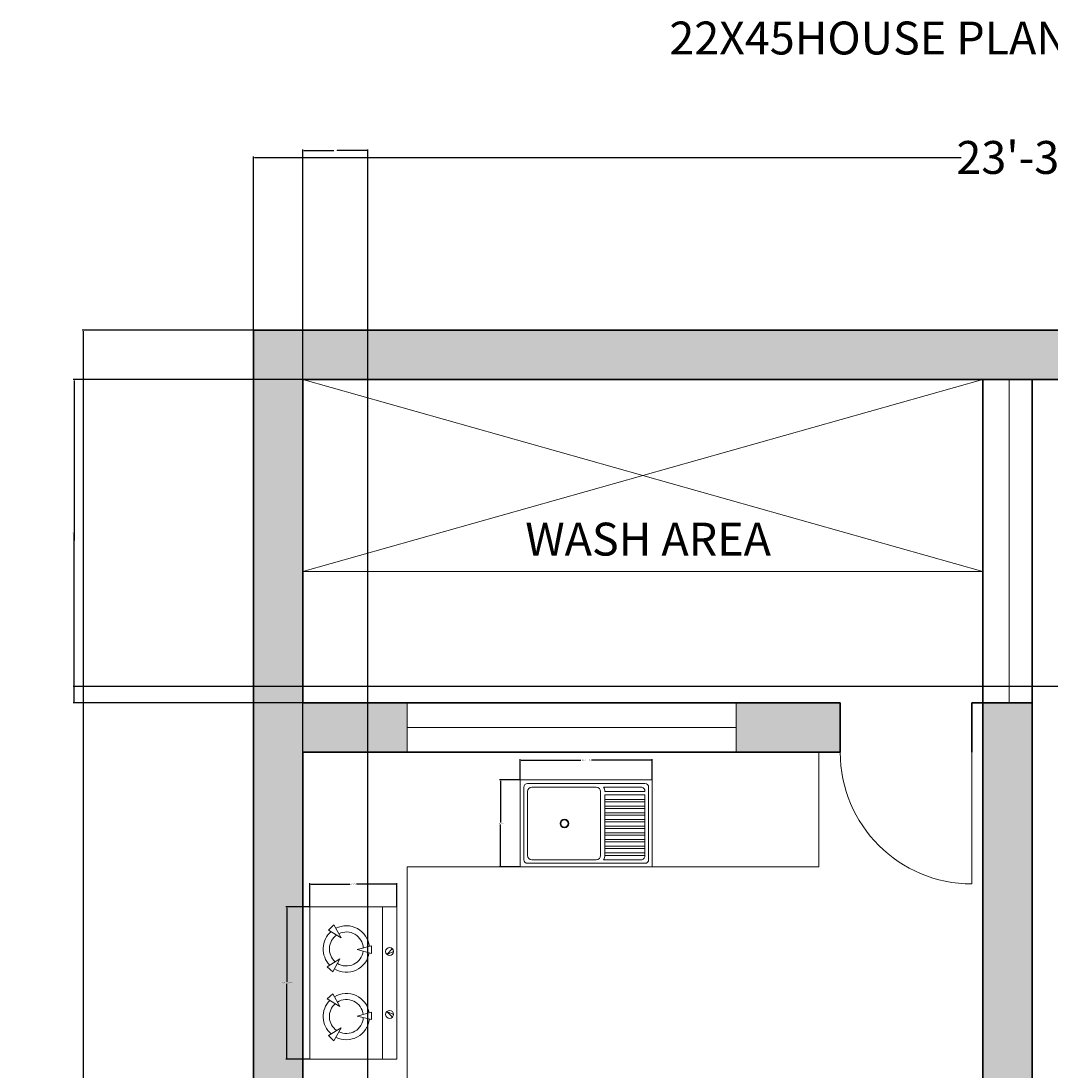
# Model space of a CAD drawing. Units: inches. Extents: x 37 to 706, y -568 to 110.
# Tile 20 of 24: x 37 to 224, y -84 to 108. Entities that reach past the tile are written whole.
import ezdxf

# ---------------------------------------------------------------- set-up
doc = ezdxf.new("R2010")
doc.units = ezdxf.units.IN
doc.header["$MEASUREMENT"] = 0
for name, color, linetype, lineweight in [('A-ANNO-DIMS', 2, 'Continuous', 18), ('A-ANNO-TEXT', 7, 'Continuous', 18), ('A-AREA-IDEN', 7, 'Continuous', 18), ('A-DOOR', 4, 'Continuous', 18), ('A-EQPM', 8, 'Continuous', 18), ('A-FLOR-CASE', 9, 'Continuous', 18), ('A-FLOR-FIXT', 9, 'Continuous', 18), ('A-FLOR-OPEN', 8, 'Continuous', 13), ('A-GLAZ', 4, 'Continuous', 18), ('A-WALL', 7, 'Continuous', 35), ('A-WALL-PATT', 252, 'Continuous', 13)]:
    doc.layers.add(name, color=color, linetype=linetype, lineweight=lineweight)
doc.styles.get("Standard").update_dxf_attribs({"font": 'arial.ttf'})
doc.dimstyles.get("Standard").update_dxf_attribs({"dimtxt": 0.18, "dimasz": 0.18, "dimexe": 0.18, "dimexo": 0.0625, "dimgap": 0.09, "dimtad": 0, "dimtih": 1, "dimtoh": 1, "dimdec": 0, "dimzin": 0, "dimdsep": 46, "dimlunit": 3, "dimtxsty": 'Standard', "dimcen": 0.09, "dimadec": 0, "dimazin": 0, "dimtfac": 1, "dimtdec": 0, "dimtofl": 0, "dimtmove": 0, "dimatfit": 3, "dimfxl": 1, "dimtolj": 1, "dimtzin": 0, "dimarcsym": 0})

# ---------------------------------------------------------------- blocks, each defined once
blk = doc.blocks.new('М12 540х820')
for p, q in [((0, 540), (-820, 540)), ((-820, 540), (-820, 0)), ((0, 0), (0, 540)), ((-797.5, 495), (-797.5, 45)), ((-45, 517.5), (-775, 517.5)), ((-775, 468), (-775, 72)), ((-347.5, 495), (-748, 495)), ((-320.5, 468), (-320.5, 72)), ((-301.7, 495), (-64.8, 495)), ((-293.7, 468), (-293.7, 472.5)), ((-293.7, 468), (-45, 468)), ((-45, 469.5), (-45, 468)), ((-22.5, 45), (-22.5, 495)), ((-293.7, 446.6), (-45, 446.6)), ((-293.7, 419.6), (-293.7, 446.6)), ((-293.7, 419.6), (-45, 419.6)), ((-293.7, 405), (-45, 405)), ((-293.7, 378), (-293.7, 405)), ((-45, 419.6), (-45, 446.6)), ((-45, 378), (-45, 405)), ((-293.7, 378), (-45, 378)), ((-293.7, 336.4), (-293.7, 363.4)), ((-293.7, 363.4), (-45, 363.4)), ((-293.7, 336.4), (-45, 336.4)), ((-45, 336.4), (-45, 363.4)), ((-293.7, 294.7), (-293.7, 321.7)), ((-293.7, 321.7), (-45, 321.7)), ((-293.7, 294.7), (-45, 294.7)), ((-293.7, 253.1), (-293.7, 280.1)), ((-293.7, 280.1), (-45, 280.1)), ((-45, 294.7), (-45, 321.7)), ((-45, 253.1), (-45, 280.1)), ((-293.7, 253.1), (-45, 253.1)), ((-293.7, 211.5), (-293.7, 238.5)), ((-293.7, 238.5), (-45, 238.5)), ((-293.7, 211.5), (-45, 211.5)), ((-293.7, 169.9), (-293.7, 196.9)), ((-293.7, 196.9), (-45, 196.9)), ((-45, 211.5), (-45, 238.5)), ((-45, 169.9), (-45, 196.9)), ((-293.7, 169.9), (-45, 169.9)), ((-293.7, 128.2), (-293.7, 155.2)), ((-293.7, 155.2), (-45, 155.2)), ((-45, 128.2), (-45, 155.2)), ((-293.7, 128.2), (-45, 128.2)), ((-293.7, 113.6), (-45, 113.6)), ((-293.7, 86.6), (-293.7, 113.6)), ((-293.7, 86.6), (-45, 86.6)), ((-293.7, 72), (-45, 72)), ((-45, 86.6), (-45, 113.6)), ((-45, 70.5), (-45, 72)), ((-820, 0), (0, 0)), ((-775, 22.5), (-45, 22.5)), ((-748, 45), (-347.5, 45)), ((-301.7, 45), (-64.8, 45))]:
    blk.add_line(p, q)
at = {"ltscale": 0.06}
for p, q in [((-820, 0), (-820, 540)), ((-820, 540), (0, 540)), ((0, 540), (0, 536.9)), ((0, 536.9), (0, 0)), ((-293.7, 446.6), (-45, 446.6)), ((-293.7, 405), (-293.7, 446.6)), ((-293.7, 363.4), (-293.7, 405)), ((-45, 446.6), (-45, 419.6)), ((-45, 419.6), (-45, 378)), ((-293.7, 321.7), (-293.7, 363.4)), ((-45, 378), (-45, 336.4)), ((-45, 336.4), (-45, 294.7)), ((-293.7, 280.1), (-293.7, 321.7)), ((-293.7, 238.5), (-293.7, 280.1)), ((-45, 294.7), (-45, 253.1)), ((-293.7, 196.9), (-293.7, 238.5)), ((-293.7, 155.2), (-293.7, 196.9)), ((-45, 253.1), (-45, 211.5)), ((-45, 211.5), (-45, 169.9)), ((-293.7, 113.6), (-293.7, 155.2)), ((-45, 169.9), (-45, 128.2)), ((-293.7, 72), (-293.7, 113.6)), ((-45, 72), (-293.7, 72)), ((-45, 128.2), (-45, 86.6)), ((-45, 86.6), (-45, 72)), ((0, 0), (-820, 0))]:
    blk.add_line(p, q, dxfattribs=at)
at = {"extrusion": (0, 0, -1)}
for centre, major_axis, start_param, end_param in [((-775, 495), (-15.9, 15.9), -0.785398, 0.785398), ((-775, 495), (-15.9, 15.9), -0.785398, 0.785398), ((-748, 468), (-19.1, -19.1), 0.785398, 2.356194), ((-748, 468), (-19.1, -19.1), 0.785398, 2.356194), ((-347.5, 468), (-19.1, 19.1), 0.785398, 2.356194), ((-347.5, 468), (-19.1, 19.1), 0.785398, 2.356194), ((-343.2, 468), (-35, 35), 1.779263, 2.356194), ((-343.2, 468), (-35, 35), 1.779263, 2.356192), ((-343.2, 468), (-35, 35), 2.356192, 2.356194), ((-72.3, 468.8), (-19.3, 19.3), 1.0328, 2.38382), ((-72.3, 468.8), (-19.3, 19.3), 1.0328, 1.064673), ((-72.3, 468.8), (-19.3, 19.3), 1.064673, 2.328569), ((-45, 495), (-15.9, -15.9), 2.356194, 3.926991), ((-45, 495), (-15.9, -15.9), 2.356194, 3.926991), ((-72.3, 468.8), (-19.3, 19.3), 2.328569, 2.38382), ((-545.5, 270), (-19.1, -19.1), 3.926991, 10.210176), ((-545.5, 270), (-19.1, -19.1), 3.926991, 10.210176), ((-545.5, 270), (-15.9, -15.9), 3.926991, 10.210176), ((-545.5, 270), (-15.9, -15.9), 3.926991, 10.210176), ((-748, 72), (-19.1, 19.1), 3.926991, 5.497787), ((-748, 72), (-19.1, 19.1), 3.926991, 5.497787), ((-347.5, 72), (-19.1, -19.1), 3.926991, 5.497787), ((-347.5, 72), (-19.1, -19.1), 3.926991, 5.497787), ((-343.2, 72), (-35, -35), 3.926991, 4.503922), ((-343.2, 72), (-35, -35), 3.926991, 4.503922), ((-72.3, 71.2), (-19.3, -19.3), 3.899365, 5.250385), ((-72.3, 71.2), (-19.3, -19.3), 3.954617, 5.218512), ((-72.3, 71.2), (-19.3, -19.3), 3.899365, 3.954617), ((-775, 45), (-15.9, -15.9), 5.497787, 7.068583), ((-775, 45), (-15.9, -15.9), 5.497787, 7.068583), ((-72.3, 71.2), (-19.3, -19.3), 5.218512, 5.250385), ((-45, 45), (-15.9, 15.9), 2.356194, 3.926991), ((-45, 45), (-15.9, 15.9), 2.356194, 3.926991)]:
    blk.add_ellipse(centre, major_axis=major_axis, ratio=1, start_param=start_param, end_param=end_param, dxfattribs=at)
blk = doc.blocks.new('*D2')
at = {"layer": 'A-ANNO-DIMS', "color": 0, "lineweight": -2, "transparency": 16777216}
for p, q in [((78.96, 51.35), (78.96, 82.95)), ((79.14, 82.77), (208.01, 82.77)), ((357.78, 82.77), (228.91, 82.77)), ((357.96, 51.35), (357.96, 82.95))]:
    blk.add_line(p, q, dxfattribs=at)
at = {"layer": 'A-ANNO-DIMS', "color": 0, "transparency": 16777216}
for points in [[(79.14, 82.8), (79.14, 82.74), (78.96, 82.77)], [(357.78, 82.8), (357.78, 82.74), (357.96, 82.77)]]:
    blk.add_solid(points, dxfattribs=at)
at = {"layer": 'Defpoints', "color": 0, "transparency": 16777216}
for p in [(357.96, 82.77), (78.96, 51.29), (357.96, 51.29)]:
    blk.add_point(p, dxfattribs=at)
at = {"layer": 'A-ANNO-DIMS', "color": 0, "transparency": 16777216, "insert": (218.46, 82.77), "char_height": 6, "attachment_point": 5}
blk.add_mtext('\\A1;23\'-3"', dxfattribs=at)
blk = doc.blocks.new('*D3')
at = {"layer": 'A-ANNO-DIMS', "color": 0, "lineweight": -2, "transparency": 16777216}
for p, q in [((78.9, 51.29), (47.67, 51.29)), ((47.85, 51.11), (47.85, -228.11)), ((47.85, -513.53), (47.85, -234.31)), ((78.9, -513.71), (47.67, -513.71))]:
    blk.add_line(p, q, dxfattribs=at)
at = {"layer": 'A-ANNO-DIMS', "color": 0, "transparency": 16777216}
for points in [[(47.82, 51.11), (47.88, 51.11), (47.85, 51.29)], [(47.82, -513.53), (47.88, -513.53), (47.85, -513.71)]]:
    blk.add_solid(points, dxfattribs=at)
at = {"layer": 'Defpoints', "color": 0, "transparency": 16777216}
for p in [(78.96, 51.29), (47.85, -513.71), (78.96, -513.71)]:
    blk.add_point(p, dxfattribs=at)
at = {"layer": 'A-ANNO-DIMS', "color": 0, "transparency": 16777216, "insert": (47.85, -231.21), "char_height": 6, "attachment_point": 5}
blk.add_mtext('\\A1;47\'-1"', dxfattribs=at)
blk = doc.blocks.new('COOKTOP-2-BURNER')
for p, q in [((13.28, 27.75), (13.28, 0)), ((3.44, 23.52), (4.41, 24.48)), ((5.73, 22.12), (3.44, 23.52)), ((4.41, 24.48), (5.73, 22.12)), ((8.68, 19.98), (11.28, 20.64)), ((11.28, 19.27), (8.68, 19.98)), ((11.28, 20.64), (11.28, 19.27)), ((3.19, 16.84), (5.49, 18.26)), ((5.49, 18.26), (4.19, 15.9)), ((4.19, 15.9), (3.19, 16.84)), ((4.19, 11.91), (3.19, 10.98)), ((5.49, 9.56), (4.19, 11.91)), ((3.19, 10.98), (5.49, 9.56)), ((11.28, 8.55), (8.68, 7.83)), ((8.68, 7.83), (11.28, 7.18)), ((11.28, 7.18), (11.28, 8.55)), ((5.73, 5.7), (3.44, 4.29)), ((3.44, 4.29), (4.41, 3.33)), ((4.41, 3.33), (5.73, 5.7))]:
    blk.add_line(p, q)
at = {"ltscale": 20}
for p, q in [((14.06, 19.09), (15.09, 20.13)), ((15.3, 19.61), (14.06, 19.09)), ((14.06, 8.66), (15.09, 7.62)), ((15.3, 8.14), (14.06, 8.66))]:
    blk.add_line(p, q, dxfattribs=at)
blk.add_lwpolyline([(0, 0), (0, 27.75), (15.86, 27.75), (15.86, 0)], close=True)
for centre in [(14.57, 19.61), (14.57, 8.14)]:
    blk.add_circle(centre, 0.73, dxfattribs=at)
for centre, radius, start, end in [((6.68, 20.07), 4.23, 131.2225, 224.1627), ((6.68, 20.07), 4.23, 6.4005, 116.769), ((6.68, 20.07), 3.1, 3.5753, 115.9207), ((6.68, 20.07), 3.1, 124.5561, 228.8027), ((6.68, 20.07), 4.23, 238.853, 350.7562), ((6.68, 20.07), 3.1, 237.9778, 353.02), ((6.68, 7.75), 4.23, 9.2438, 121.147), ((6.68, 7.75), 4.23, 135.8373, 228.7775), ((6.68, 7.75), 3.1, 131.1973, 235.4439), ((6.68, 7.75), 3.1, 6.98, 122.0222), ((6.68, 7.75), 4.23, 243.231, 353.5995), ((6.68, 7.75), 3.1, 244.0793, 356.4247)]:
    blk.add_arc(centre, radius, start, end)
blk = doc.blocks.new('WIN-60')
for p, q in [((60, 9), (0, 9)), ((0, 9), (0, 0)), ((60, 0), (60, 9)), ((60, 4.5), (0, 4.5)), ((0, 0), (60, 0))]:
    blk.add_line(p, q)
blk = doc.blocks.new('DOOR-SWING-24')
blk.add_line((0, 0), (0, 24))
blk.add_arc((0, 0), 24, 0, 90)
blk = doc.blocks.new('*D27')
at = {"layer": 'A-ANNO-DIMS', "color": 0, "lineweight": -2, "transparency": 16777216}
for p, q in [((127.58, -30.69), (127.58, -26.96)), ((127.76, -27.14), (138.66, -27.14)), ((151.49, -27.14), (140.59, -27.14)), ((151.67, -30.69), (151.67, -26.96))]:
    blk.add_line(p, q, dxfattribs=at)
at = {"layer": 'A-ANNO-DIMS', "color": 0, "transparency": 16777216}
for points in [[(127.76, -27.11), (127.76, -27.17), (127.58, -27.14)], [(151.49, -27.11), (151.49, -27.17), (151.67, -27.14)]]:
    blk.add_solid(points, dxfattribs=at)
at = {"layer": 'Defpoints', "color": 0, "transparency": 16777216}
for p in [(151.67, -27.14), (127.58, -30.75), (151.67, -30.75)]:
    blk.add_point(p, dxfattribs=at)
at = {"layer": 'A-ANNO-DIMS', "color": 0, "transparency": 16777216, "insert": (139.63, -27.14), "char_height": 0.18, "attachment_point": 5}
blk.add_mtext('\\A1;SINK 2\'-0" TYP.', dxfattribs=at)
blk = doc.blocks.new('*D28')
at = {"layer": 'A-ANNO-DIMS', "color": 0, "lineweight": -2, "transparency": 16777216}
for p, q in [((127.52, -30.75), (123.79, -30.75)), ((123.97, -30.93), (123.97, -38.5)), ((123.97, -46.43), (123.97, -38.86)), ((127.52, -46.61), (123.79, -46.61))]:
    blk.add_line(p, q, dxfattribs=at)
at = {"layer": 'A-ANNO-DIMS', "color": 0, "transparency": 16777216}
for points in [[(123.94, -30.93), (124, -30.93), (123.97, -30.75)], [(123.94, -46.43), (124, -46.43), (123.97, -46.61)]]:
    blk.add_solid(points, dxfattribs=at)
at = {"layer": 'Defpoints', "color": 0, "transparency": 16777216}
for p in [(123.97, -30.75), (127.58, -30.75), (127.58, -46.61)]:
    blk.add_point(p, dxfattribs=at)
at = {"layer": 'A-ANNO-DIMS', "color": 0, "transparency": 16777216, "insert": (123.97, -38.68), "char_height": 0.18, "attachment_point": 5}
blk.add_mtext('\\A1;1\'-4" TYP.', dxfattribs=at)
blk = doc.blocks.new('*D33')
at = {"layer": 'A-ANNO-DIMS', "color": 0, "lineweight": -2, "transparency": 16777216}
for p, q in [((89.14, -53.89), (84.86, -53.89)), ((85.04, -54.07), (85.04, -67.58)), ((85.04, -81.46), (85.04, -67.95)), ((89.14, -81.64), (84.86, -81.64))]:
    blk.add_line(p, q, dxfattribs=at)
at = {"layer": 'A-ANNO-DIMS', "color": 0, "transparency": 16777216}
for points in [[(85.01, -54.07), (85.07, -54.07), (85.04, -53.89)], [(85.01, -81.46), (85.07, -81.46), (85.04, -81.64)]]:
    blk.add_solid(points, dxfattribs=at)
at = {"layer": 'Defpoints', "color": 0, "transparency": 16777216}
for p in [(85.04, -53.89), (89.2, -53.89), (89.2, -81.64)]:
    blk.add_point(p, dxfattribs=at)
at = {"layer": 'A-ANNO-DIMS', "color": 0, "transparency": 16777216, "insert": (85.04, -67.76), "char_height": 0.18, "attachment_point": 5}
blk.add_mtext('\\A1;HOB 2\'-3 1/2" TYP.', dxfattribs=at)
blk = doc.blocks.new('*D34')
at = {"layer": 'A-ANNO-DIMS', "color": 0, "lineweight": -2, "transparency": 16777216}
for p, q in [((89.2, -53.83), (89.2, -49.55)), ((89.38, -49.73), (96.5, -49.73)), ((104.88, -49.73), (97.76, -49.73)), ((105.06, -53.83), (105.06, -49.55))]:
    blk.add_line(p, q, dxfattribs=at)
at = {"layer": 'A-ANNO-DIMS', "color": 0, "transparency": 16777216}
for points in [[(89.38, -49.7), (89.38, -49.76), (89.2, -49.73)], [(104.88, -49.7), (104.88, -49.76), (105.06, -49.73)]]:
    blk.add_solid(points, dxfattribs=at)
at = {"layer": 'Defpoints', "color": 0, "transparency": 16777216}
for p in [(105.06, -49.73), (89.2, -53.89), (105.06, -53.89)]:
    blk.add_point(p, dxfattribs=at)
at = {"layer": 'A-ANNO-DIMS', "color": 0, "transparency": 16777216, "insert": (97.13, -49.73), "char_height": 0.18, "attachment_point": 5}
blk.add_mtext('\\A1;1\'-4" TYP.', dxfattribs=at)
blk = doc.blocks.new('*D41')
at = {"layer": 'A-ANNO-DIMS', "color": 0, "lineweight": -2, "transparency": 16777216}
for p, q in [((87.9, 42.29), (46.03, 42.29)), ((46.21, 42.11), (46.21, 12.97)), ((46.21, -16.53), (46.21, 12.61)), ((87.9, -16.71), (46.03, -16.71))]:
    blk.add_line(p, q, dxfattribs=at)
at = {"layer": 'A-ANNO-DIMS', "color": 0, "transparency": 16777216}
for points in [[(46.18, 42.11), (46.24, 42.11), (46.21, 42.29)], [(46.18, -16.53), (46.24, -16.53), (46.21, -16.71)]]:
    blk.add_solid(points, dxfattribs=at)
at = {"layer": 'Defpoints', "color": 0, "transparency": 16777216}
for p in [(87.96, 42.29), (46.21, -16.71), (87.96, -16.71)]:
    blk.add_point(p, dxfattribs=at)
at = {"layer": 'A-ANNO-DIMS', "color": 0, "transparency": 16777216, "insert": (46.21, 12.79), "char_height": 0.18, "attachment_point": 5}
blk.add_mtext('\\A1;4\'-11"', dxfattribs=at)
blk = doc.blocks.new('*D42')
at = {"layer": 'A-ANNO-DIMS', "color": 0, "lineweight": -2, "transparency": 16777216}
for p, q in [((402.9, 42.29), (46.03, 42.29)), ((46.21, 42.11), (46.21, 14.47)), ((46.21, -13.53), (46.21, 14.11)), ((402.9, -13.71), (46.03, -13.71))]:
    blk.add_line(p, q, dxfattribs=at)
at = {"layer": 'A-ANNO-DIMS', "color": 0, "transparency": 16777216}
for points in [[(46.18, 42.11), (46.24, 42.11), (46.21, 42.29)], [(46.18, -13.53), (46.24, -13.53), (46.21, -13.71)]]:
    blk.add_solid(points, dxfattribs=at)
at = {"layer": 'Defpoints', "color": 0, "transparency": 16777216}
for p in [(402.96, 42.29), (46.21, -13.71), (402.96, -13.71)]:
    blk.add_point(p, dxfattribs=at)
at = {"layer": 'A-ANNO-DIMS', "color": 0, "transparency": 16777216, "insert": (46.21, 14.29), "char_height": 0.18, "attachment_point": 5}
blk.add_mtext('\\A1;4\'-8"', dxfattribs=at)
blk = doc.blocks.new('*D60')
at = {"layer": 'A-ANNO-DIMS', "color": 0, "lineweight": -2, "transparency": 16777216}
for p, q in [((87.96, -142.65), (87.96, 84.22)), ((88.14, 84.04), (93.57, 84.04)), ((99.64, 84.04), (94.21, 84.04)), ((99.82, -176.5), (99.82, 84.22))]:
    blk.add_line(p, q, dxfattribs=at)
at = {"layer": 'A-ANNO-DIMS', "color": 0, "transparency": 16777216}
for points in [[(88.14, 84.07), (88.14, 84.01), (87.96, 84.04)], [(99.64, 84.07), (99.64, 84.01), (99.82, 84.04)]]:
    blk.add_solid(points, dxfattribs=at)
at = {"layer": 'Defpoints', "color": 0, "transparency": 16777216}
for p in [(99.82, 84.04), (87.96, -142.71), (99.82, -176.56)]:
    blk.add_point(p, dxfattribs=at)
at = {"layer": 'A-ANNO-DIMS', "color": 0, "transparency": 16777216, "insert": (93.89, 84.04), "char_height": 0.18, "attachment_point": 5}
blk.add_mtext('\\A1;1\'-0"', dxfattribs=at)

msp = doc.modelspace()

# ---------------------------------------------------------------- hatches: boundary and pattern name
at = {"layer": 'A-WALL-PATT'}
h = msp.add_hatch(color=256, dxfattribs=at)
h.dxf.hatch_style = 1
h.paths.add_polyline_path([(220.96, -351.71), (211.96, -351.71), (211.96, -513.71), (254.96, -513.71), (254.96, -504.71), (220.96, -504.71)], flags=17)
h.paths.add_polyline_path([(220.96, -294.71), (211.96, -294.71), (211.96, -303.71), (220.96, -303.71)], flags=17)
h.paths.add_polyline_path([(175.96, -294.71), (155.87, -294.71), (155.87, -303.71), (155.96, -303.71), (175.96, -303.71)], flags=17)
h.paths.add_polyline_path([(220.96, -16.71), (211.96, -16.71), (211.96, -142.71), (220.96, -142.71)], flags=17)
h.paths.add_polyline_path([(357.96, 51.29), (78.96, 51.29), (78.96, -513.71), (87.96, -513.71), (87.96, -303.71), (95.87, -303.71), (95.87, -294.71), (87.96, -294.71), (87.96, -142.71), (187.96, -142.71), (187.96, -133.71), (87.96, -133.71), (87.96, -25.71), (106.96, -25.71), (106.96, -16.71), (87.96, -16.71), (87.96, 42.29), (348.96, 42.29), (348.96, 17.13), (348.96, -133.71), (246.96, -133.71), (246.96, -142.71), (348.96, -142.71), (348.96, -294.71), (251.96, -294.71), (251.96, -303.71), (348.96, -303.71), (348.96, -351.71), (260.96, -351.71), (260.96, -329.71), (251.96, -329.71), (251.96, -360.71), (327.45, -360.71), (348.96, -360.71), (348.96, -504.71), (314.96, -504.71), (314.96, -513.71), (357.96, -513.71)])
h.paths.add_polyline_path([(416.96, -303.71), (402.96, -303.71), (402.96, -151.71), (478.96, -151.71), (478.96, -142.71), (402.96, -142.71), (402.96, -22.71), (409.96, -22.71), (409.96, -13.71), (402.96, -13.71), (402.96, 42.29), (663.96, 42.29), (663.96, -303.71), (566.96, -303.71), (566.96, -312.71), (663.96, -312.71), (663.96, -360.71), (575.96, -360.71), (575.96, -338.71), (566.96, -338.71), (566.96, -360.71), (566.96, -369.71), (642.45, -369.71), (663.96, -369.71), (663.96, -513.71), (629.96, -513.71), (629.96, -522.71), (672.96, -522.71), (672.96, 51.29), (393.96, 51.29), (393.96, -522.71), (402.96, -522.71), (402.96, -312.71), (416.96, -312.71)])
h.paths.add_polyline_path([(490.96, -303.71), (476.96, -303.71), (476.96, -312.71), (490.96, -312.71)], flags=17)
h.paths.add_polyline_path([(535.96, -303.71), (526.96, -303.71), (526.96, -312.71), (535.96, -312.71)], flags=17)
h.paths.add_polyline_path([(535.96, -369.71), (526.96, -369.71), (526.96, -522.71), (569.96, -522.71), (569.96, -513.71), (535.96, -513.71)], flags=17)
h.paths.add_polyline_path([(511.96, -13.71), (502.96, -13.71), (502.96, -151.71), (511.96, -151.71)], flags=17)
h.paths.add_polyline_path([(651.54, -142.71), (651.54, -120.18), (642.54, -120.18), (642.54, -142.71), (550.54, -142.71), (550.54, -120.71), (541.54, -120.71), (541.54, -142.71), (537.96, -142.71), (537.96, -151.71), (651.54, -151.71)], flags=17)
h.paths.add_polyline_path([(651.54, -85.71), (541.54, -85.71), (541.54, -94.71), (651.54, -94.71)], flags=17)
h.paths.add_polyline_path([(476.96, -13.71), (469.96, -13.71), (469.96, -22.71), (476.96, -22.71)], flags=17)
h.paths.add_polyline_path([(185.96, -16.71), (166.96, -16.71), (166.96, -25.71), (185.96, -25.71)], flags=17)
h.paths.add_polyline_path([(168.91, -414.72), (214.62, -414.72), (214.62, -392.33), (168.91, -392.33)], flags=25)

# ---------------------------------------------------------------- linework, layer by layer
at = {"layer": 'A-FLOR-CASE'}
for p, q in [((182.04, -25.71), (182.04, -46.61)), ((182.04, -46.61), (106.97, -46.61)), ((106.97, -46.61), (106.97, -133.71))]:
    msp.add_line(p, q, dxfattribs=at)
at = {"layer": 'A-FLOR-OPEN'}
for p, q in [((87.96, 42.29), (211.96, 7.29)), ((211.96, 42.29), (87.96, 7.29)), ((87.96, 7.29), (211.96, 7.29))]:
    msp.add_line(p, q, dxfattribs=at)
at = {"layer": 'A-GLAZ'}
msp.add_line((216.74, -16.71), (216.74, 42.29), dxfattribs=at)
at = {"layer": 'A-WALL'}
for p, q in [((78.96, 51.29), (78.96, -513.71)), ((78.96, 51.29), (357.96, 51.29)), ((87.96, 42.29), (348.96, 42.29)), ((87.96, 42.29), (87.96, -16.71)), ((211.96, 42.29), (211.96, -142.71)), ((220.96, 42.29), (220.96, -142.71)), ((87.96, -16.71), (185.96, -16.71)), ((185.96, -16.71), (185.96, -25.71)), ((209.96, -16.71), (209.96, -25.71)), ((209.96, -16.71), (220.96, -16.71)), ((87.96, -25.71), (185.96, -25.71)), ((87.96, -25.71), (87.96, -133.71))]:
    msp.add_line(p, q, dxfattribs=at)

# ---------------------------------------------------------------- block references
at = {"layer": 'A-DOOR', "rotation": 180}
msp.add_blockref('DOOR-SWING-24', (209.96, -25.71), dxfattribs=at)
at = {"layer": 'A-EQPM'}
msp.add_blockref('COOKTOP-2-BURNER', (89.2, -81.64), dxfattribs=at)
at = {"layer": 'A-FLOR-FIXT', "xscale": 0.0293785137493104, "yscale": 0.0293785137493104, "zscale": 0.0293785137493104}
msp.add_blockref('М12 540х820', (151.67, -46.61), dxfattribs=at)
at = {"layer": 'A-GLAZ'}
msp.add_blockref('WIN-60', (106.96, -25.71), dxfattribs=at)

# ---------------------------------------------------------------- texts
at = {"layer": 'A-ANNO-TEXT', "insert": (154.79, 107.55), "char_height": 6, "attachment_point": 1}
msp.add_mtext('22X45HOUSE PLAN NORTH FACING', dxfattribs=at)
at = {"layer": 'A-AREA-IDEN', "insert": (128.51, 16.17), "char_height": 6, "attachment_point": 1}
msp.add_mtext('WASH AREA', dxfattribs=at)

# ---------------------------------------------------------------- dimensions: what is measured, and where the dimension line sits
at = {"layer": 'A-ANNO-DIMS'}
for base, p1, p2, override, picture, middle in [((357.96, 82.77), (78.96, 51.29), (357.96, 51.29), {"dimtxt": 6, "dimclrd": 0, "dimclre": 0, "dimclrt": 0}, '*D2', (218.46, 82.77)), ((99.82, 84.04), (87.96, -142.71), (99.82, -176.56), {"dimdec": 1, "dimlfac": 1, "dimrnd": 0, "dimzin": 1, "dimdsep": 46, "dimlunit": 4, "dimfrac": 2}, '*D60', (93.89, 84.04))]:
    dim = msp.add_linear_dim(base=base, p1=p1, p2=p2, dimstyle='Standard', override=override, dxfattribs=at)
    dim.commit()
    dim.dimension.update_dxf_attribs({"geometry": picture, "text_midpoint": middle})
for base, p1, p2, override, picture, middle in [((47.85, -513.71), (78.96, 51.29), (78.96, -513.71), {"dimtxt": 6, "dimclrd": 0, "dimclre": 0, "dimclrt": 0}, '*D3', (47.85, -231.21)), ((46.21, -16.71), (87.96, 42.29), (87.96, -16.71), {"dimdec": 1, "dimlfac": 1, "dimrnd": 0, "dimzin": 1, "dimdsep": 46, "dimlunit": 4, "dimfrac": 2}, '*D41', (46.21, 12.79)), ((46.21, -13.71), (402.96, 42.29), (402.96, -13.71), {"dimdec": 1, "dimlfac": 1, "dimrnd": 0, "dimzin": 1, "dimdsep": 46, "dimlunit": 4, "dimfrac": 2}, '*D42', (46.21, 14.29))]:
    dim = msp.add_linear_dim(base=base, p1=p1, p2=p2, angle=90, dimstyle='Standard', override=override, dxfattribs=at)
    dim.commit()
    dim.dimension.update_dxf_attribs({"geometry": picture, "text_midpoint": middle})
for base, p1, p2, text, picture, middle in [((151.67, -27.14), (127.58, -30.75), (151.67, -30.75), 'SINK <> TYP.', '*D27', (139.63, -27.14)), ((105.06, -49.73), (89.2, -53.89), (105.06, -53.89), '<> TYP.', '*D34', (97.13, -49.73))]:
    dim = msp.add_linear_dim(base=base, p1=p1, p2=p2, text=text, dimstyle='Standard', override={"dimdec": 1, "dimlfac": 1, "dimrnd": 0, "dimzin": 1, "dimdsep": 46, "dimlunit": 4, "dimfrac": 2}, dxfattribs=at)
    dim.commit()
    dim.dimension.update_dxf_attribs({"geometry": picture, "text_midpoint": middle})
for base, p1, p2, text, picture, middle in [((123.97, -30.75), (127.58, -46.61), (127.58, -30.75), '<> TYP.', '*D28', (123.97, -38.68)), ((85.0412, -53.891), (89.2032, -81.638), (89.2032, -53.891), 'HOB <> TYP.', '*D33', (85.0412, -67.7645))]:
    dim = msp.add_linear_dim(base=base, p1=p1, p2=p2, angle=90, text=text, dimstyle='Standard', override={"dimdec": 1, "dimlfac": 1, "dimrnd": 0, "dimzin": 1, "dimdsep": 46, "dimlunit": 4, "dimfrac": 2}, dxfattribs=at)
    dim.commit()
    dim.dimension.update_dxf_attribs({"geometry": picture, "text_midpoint": middle})

doc.saveas('drawing.dxf')
